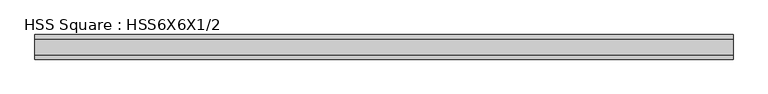
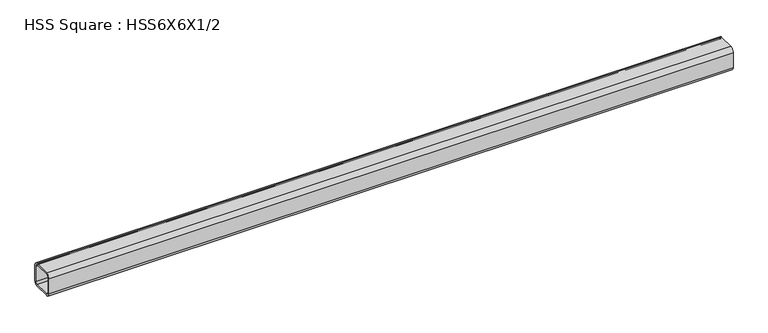
"""IFC4 building model written with IfcOpenShell, lengths in millimetres: member geometry, HSS Square : HSS6X6X1/2."""

from ifc_helpers import new_model, si_unit, point, frame, frame_2d, origin, place, context, project, spatial, polyline, circle_curve, trimmed, segment, composite_curve, outline, extrude, source, transform, mapped, element, save


def hss_square_hss6x6x1_2_008024fe(model_context):
    return source(origin(), model_context, "Body", "SweptSolid", [
        extrude(outline(composite_curve([segment(polyline([(76.2, 50.8), (76.2, -50.8)]), True, "CONTINUOUS"), segment(trimmed(circle_curve(frame_2d((50.8, -50.8)), 25.4), [point((76.2, -50.8))], [point((50.8, -76.2))], False, "CARTESIAN"), True, "CONTINUOUS"), segment(polyline([(50.8, -76.2), (-50.8, -76.2)]), True, "CONTINUOUS"), segment(trimmed(circle_curve(frame_2d((-50.8, -50.8)), 25.4), [point((-50.8, -76.2))], [point((-76.2, -50.8))], False, "CARTESIAN"), True, "CONTINUOUS"), segment(polyline([(-76.2, -50.8), (-76.2, 50.8)]), True, "CONTINUOUS"), segment(trimmed(circle_curve(frame_2d((-50.8, 50.8)), 25.4), [point((-76.2, 50.8))], [point((-50.8, 76.2))], False, "CARTESIAN"), True, "CONTINUOUS"), segment(polyline([(-50.8, 76.2), (50.8, 76.2)]), True, "CONTINUOUS"), segment(trimmed(circle_curve(frame_2d((50.8, 50.8)), 25.4), [point((50.8, 76.2))], [point((76.2, 50.8))], False, "CARTESIAN"), True, "CONTINUOUS")], self_intersect=False), holes=[composite_curve([segment(trimmed(circle_curve(frame_2d((-50.8, 50.8)), 12.7), [point((-50.8, 63.5))], [point((-63.5, 50.8))], True, "CARTESIAN"), True, "CONTINUOUS"), segment(polyline([(-63.5, 50.8), (-63.5, -50.8)]), True, "CONTINUOUS"), segment(trimmed(circle_curve(frame_2d((-50.8, -50.8)), 12.7), [point((-63.5, -50.8))], [point((-50.8, -63.5))], True, "CARTESIAN"), True, "CONTINUOUS"), segment(polyline([(-50.8, -63.5), (50.8, -63.5)]), True, "CONTINUOUS"), segment(trimmed(circle_curve(frame_2d((50.8, -50.8)), 12.7), [point((50.8, -63.5))], [point((63.5, -50.8))], True, "CARTESIAN"), True, "CONTINUOUS"), segment(polyline([(63.5, -50.8), (63.5, 50.8)]), True, "CONTINUOUS"), segment(trimmed(circle_curve(frame_2d((50.8, 50.8)), 12.7), [point((63.5, 50.8))], [point((50.8, 63.5))], True, "CARTESIAN"), True, "CONTINUOUS"), segment(polyline([(50.8, 63.5), (-50.8, 63.5)]), True, "CONTINUOUS")], self_intersect=False)]), frame((-2097.5113984, 0.0, 0.0), z_axis=(1.0, 0.0, 0.0), x_axis=(0.0, 1.0, 0.0)), (0.0, 0.0, 1.0), 4321.0754934),
    ])


if __name__ == "__main__":
    model = new_model("IFC4")
    model_context = context("Model", 3, world=origin())
    ifc_project = project(units=[si_unit("LENGTHUNIT", "METRE", prefix="MILLI")], contexts=[model_context])
    site = spatial("IfcSite", under=ifc_project)
    building = spatial("IfcBuilding", under=site)
    placement = place(None, origin())
    hss_square_hss6x6x1_2_shape = hss_square_hss6x6x1_2_008024fe(model_context)
    element("IfcMember", 1, ObjectType="HSS Square : HSS6X6X1/2", at=placement, inside=building, context=model_context, shape_type="MappedRepresentation", body=[
        mapped(hss_square_hss6x6x1_2_shape, transform((0.0, 0.0, 0.0), x_axis=(1.0, 0.0, 0.0), y_axis=(0.0, 1.0, 0.0), z_axis=(0.0, 0.0, 1.0))),
    ])
    save(model, "model.ifc")

# Revit data of these elements
# Type "HSS Square : HSS6X6X1/2"
#   Section Name Key = "HSS 6X6X1/2"
#   Assembly Code = "B10"
#   Width = 6.000"
#   Wall Nominal Thickness = 0.500"
#   Wall Design Thickness = 0.465"
#   Torsional Moment of Inertia = 81.10 in⁴
#   Torsional Modulus = 28.10 in³
#   Section Area = 9.74 in²
#   Plastic Modulus weak axis = 19.80 in³
#   Plastic Modulus strong axis = 19.80 in³
#   Outer Fillet = 1.000"
#   Nominal Weight = 35.24 lbf/ft
#   Moment of Inertia weak axis = 48.30 in⁴
#   Moment of Inertia strong axis = 48.30 in⁴
#   Inner Fillet = 0.500"
#   Height = 6.000"
#   Elastic Modulus weak axis = 16.10 in³
#   Elastic Modulus strong axis = 16.10 in³
#   Centroid Vertical = 3.000"
#   Centroid Horizontal = 3.000"
#   Length [instance default] = 5' - 0"
#   Structural Material [instance default] = Steel ASTM A500, Grade B, Rectangular and Square
#   Principal Axes Angle = 0
# Element 1 (IfcMember, "HSS Square : HSS6X6X1/2")
#   Structural Material = Steel ASTM A992
#   Materials on its faces: "Steel ASTM A992"
# Materials
#   "Steel ASTM A500, Grade B, Rectangular and Square": class "Metal", colour RGB 199 199 199, transparency 0, Description = "Carbon steel", Cost = 0
#   "Steel ASTM A992": class "Metal", colour RGB 199 199 199, transparency 0, Description = "Structural steel 50ksi", Cost = 0
